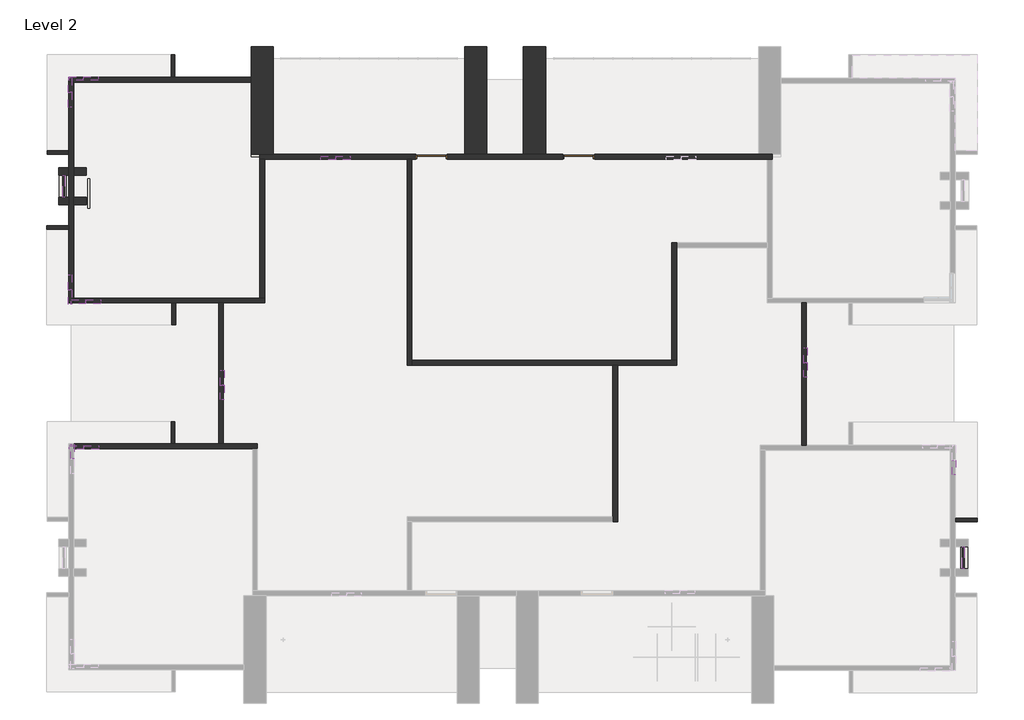
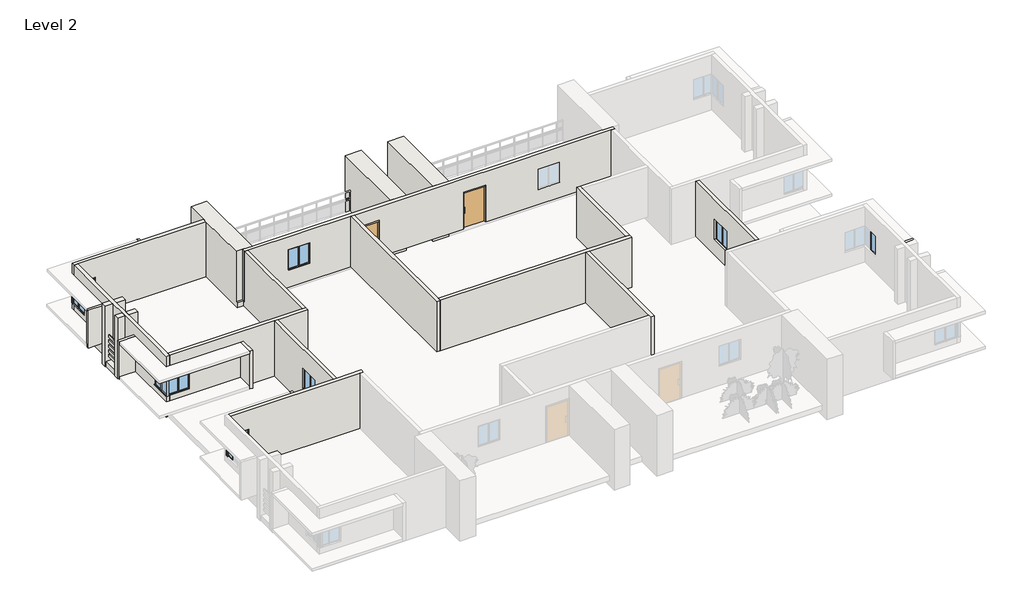
# One storey, part 2 of 4: 37 walls, 18 windows, 2 doors.
"""IFC4 building model written with IfcOpenShell, lengths in millimetres."""

from ifc_helpers import new_model, si_unit, frame, origin, place, context, project, spatial, polyline, outline, extrude, faceted_brep, transform, mapped, element, save
from components import door_15d3c954, window_20ff4747

model = new_model("IFC4")

# Units and contexts
model_context = context("Model", 3, world=origin())
ifc_project = project(units=[si_unit("LENGTHUNIT", "METRE", prefix="MILLI")], contexts=[model_context])

# Site, building, storey
site = spatial("IfcSite", under=ifc_project)
building = spatial("IfcBuilding", under=site)
storey = spatial("IfcBuildingStorey", under=building, Name="Level 2", Elevation=3048.0)

# Doors
placement = place(None, origin())
door_shape = door_15d3c954(model_context)
element("IfcDoor", 1, ObjectType="Door-Passage-Single-Flush-Dbl_Acting : 48\" x 96\"", at=placement, inside=storey, context=model_context, shape_type="MappedRepresentation", body=[
    mapped(door_shape, transform((6249.0520665, 12804.5205944, 3657.6), x_axis=(1.0, 0.0, 0.0), y_axis=(0.0, 1.0, 0.0), z_axis=(0.0, 0.0, 1.0))),
])
element("IfcDoor", 2, ObjectType="Door-Passage-Single-Flush-Dbl_Acting : 48\" x 96\"", at=placement, inside=storey, context=model_context, shape_type="MappedRepresentation", body=[
    mapped(door_shape, transform((153.0520665, 12804.5205944, 3657.6), x_axis=(1.0, 0.0, 0.0), y_axis=(0.0, 1.0, 0.0), z_axis=(0.0, 0.0, 1.0))),
])

# Walls
element("IfcWall", 3, ObjectType="Generic - 1'", at=placement, inside=storey, context=model_context, shape_type="SweptSolid", body=[
    extrude(outline(polyline([(-14151.7972154, 12048.8705944), (-14667.8479335, 12048.8705944), (-14667.8479335, 12353.6705944), (-14151.7972154, 12353.6705944), (-14151.7972154, 12048.8705944)])), frame((0.0, 0.0, 3048.0), z_axis=(0.0, 0.0, 1.0), x_axis=(1.0, 0.0, 0.0)), (0.0, 0.0, 1.0), 3657.6),
])
element("IfcWall", 4, ObjectType="Generic - 1'", at=placement, inside=storey, context=model_context, shape_type="Brep", body=[
    faceted_brep([(-14871.0479335, 12353.6705944, 3048.0), (-15302.1394029, 12353.6705944, 3048.0), (-15302.1394029, 12353.6705944, 6705.6), (-14871.0479335, 12353.6705944, 6705.6), (-14871.0479335, 12048.8705944, 3048.0), (-14871.0479335, 12048.8705944, 6705.6), (-15302.1394029, 12048.8705944, 6705.6), (-15302.1394029, 12048.8705944, 3048.0), (-15277.0936682, 12048.8705944, 3048.0), (-14972.2936682, 12048.8705944, 3048.0)], [[[0, 1, 2, 3]], [[4, 5, 6, 7, 8, 9]], [[1, 0, 4, 9, 8, 7]], [[2, 1, 7, 6]], [[3, 2, 6, 5]], [[0, 3, 5, 4]]]),
])
element("IfcWall", 5, ObjectType="Generic - 1'", at=placement, inside=storey, context=model_context, shape_type="SweptSolid", body=[
    extrude(outline(polyline([(-14151.7972154, 10829.6705944), (-14667.8479335, 10829.6705944), (-14667.8479335, 11134.4705944), (-14151.7972154, 11134.4705944), (-14151.7972154, 10829.6705944)])), frame((0.0, 0.0, 3048.0), z_axis=(0.0, 0.0, 1.0), x_axis=(1.0, 0.0, 0.0)), (0.0, 0.0, 1.0), 3657.6),
])
element("IfcWall", 6, ObjectType="Generic - 1'", at=placement, inside=storey, context=model_context, shape_type="Brep", body=[
    faceted_brep([(-14871.0479335, 11134.4705944, 3048.0), (-14972.2936682, 11134.4705944, 3048.0), (-15277.0936682, 11134.4705944, 3048.0), (-15302.1394029, 11134.4705944, 3048.0), (-15302.1394029, 11134.4705944, 6705.6), (-14871.0479335, 11134.4705944, 6705.6), (-14871.0479335, 10829.6705944, 3048.0), (-14871.0479335, 10829.6705944, 6705.6), (-15302.1394029, 10829.6705944, 6705.6), (-15302.1394029, 10829.6705944, 3048.0)], [[[0, 1, 2, 3, 4, 5]], [[6, 7, 8, 9]], [[3, 2, 1, 0, 6, 9]], [[4, 3, 9, 8]], [[5, 4, 8, 7]], [[0, 5, 7, 6]]]),
])
element("IfcWall", 7, ObjectType="Generic - 2'", at=placement, inside=storey, context=model_context, shape_type="SweptSolid", body=[
    extrude(outline(polyline([(22069.7857703, -4257.9294056), (22069.7857703, -3343.5294056), (22374.5857703, -3343.5294056), (22374.5857703, -4257.9294056), (22069.7857703, -4257.9294056)])), frame((0.0, 0.0, 3048.0), z_axis=(0.0, 0.0, 1.0), x_axis=(1.0, 0.0, 0.0)), (0.0, 0.0, 1.0), 304.8),
])
element("IfcWall", 8, ObjectType="Generic - 2'", at=placement, inside=storey, context=model_context, shape_type="SweptSolid", body=[
    extrude(outline(polyline([(-15277.0936682, 11134.4705944), (-15277.0936682, 12048.8705944), (-14972.2936682, 12048.8705944), (-14972.2936682, 11134.4705944), (-15277.0936682, 11134.4705944)])), frame((0.0, 0.0, 3048.0), z_axis=(0.0, 0.0, 1.0), x_axis=(1.0, 0.0, 0.0)), (0.0, 0.0, 1.0), 304.8),
])
element("IfcWall", 9, ObjectType="Generic - 3'", at=placement, inside=storey, context=model_context, shape_type="SweptSolid", body=[
    extrude(outline(polyline([(2439.0520665, 17382.8705944), (2439.0520665, 12912.4705944), (1524.6520665, 12912.4705944), (1524.6520665, 17382.8705944), (2439.0520665, 17382.8705944)])), frame((0.0, 0.0, 3048.0), z_axis=(0.0, 0.0, 1.0), x_axis=(1.0, 0.0, 0.0)), (0.0, 0.0, 1.0), 3657.6),
])
element("IfcWall", 10, ObjectType="Generic - 3'", at=placement, inside=storey, context=model_context, shape_type="SweptSolid", body=[
    extrude(outline(polyline([(4877.4520665, 17382.8705944), (4877.4520665, 12912.4705944), (3963.0520665, 12912.4705944), (3963.0520665, 17382.8705944), (4877.4520665, 17382.8705944)])), frame((0.0, 0.0, 3048.0), z_axis=(0.0, 0.0, 1.0), x_axis=(1.0, 0.0, 0.0)), (0.0, 0.0, 1.0), 3657.6),
])
element("IfcWall", 11, ObjectType="Generic - 3'", at=placement, inside=storey, context=model_context, shape_type="Brep", body=[
    faceted_brep([(-6400.1479335, 12810.8705944, 3048.0), (-6400.1479335, 17382.8705944, 3048.0), (-6400.1479335, 17382.8705944, 6705.6), (-6400.1479335, 12912.4705944, 6705.6), (-6400.1479335, 12912.4705944, 3657.6), (-6400.1479335, 12810.8705944, 3657.6), (-7314.5479335, 12810.8705944, 3048.0), (-7314.5479335, 12810.8705944, 3657.6), (-7314.5479335, 12912.4705944, 3657.6), (-7314.5479335, 12912.4705944, 6705.6), (-7314.5479335, 15904.9548886, 6705.6), (-7314.5479335, 16108.1548886, 6705.6), (-7314.5479335, 17382.8705944, 6705.6), (-7314.5479335, 17382.8705944, 3048.0), (-7314.5479335, 16108.1548886, 3048.0), (-7314.5479335, 15904.9548886, 3048.0), (-6755.7479335, 12810.8705944, 3048.0), (-6958.9479335, 12810.8705944, 3048.0), (-6958.9479335, 12912.4705944, 6705.6), (-6755.7479335, 12810.8705944, 3657.6), (-6958.9479335, 12810.8705944, 3657.6), (-6958.9479335, 12912.4705944, 3657.6)], [[[0, 1, 2, 3, 4, 5]], [[6, 7, 8, 9, 10, 11, 12, 13, 14, 15]], [[1, 0, 16, 17, 6, 15, 14, 13]], [[2, 1, 13, 12]], [[3, 2, 12, 11, 10, 9, 18]], [[0, 5, 19, 20, 7, 6, 17, 16]], [[4, 21, 8, 7, 20, 19, 5]], [[4, 3, 18, 9, 8, 21]]]),
])
element("IfcWall", 12, ObjectType="Generic - 5\"", at=placement, inside=storey, context=model_context, shape_type="SweptSolid", body=[
    extrude(outline(polyline([(-14084.4224108, 10677.2705944), (-14084.4224108, 11896.4705944), (-14008.2224108, 11896.4705944), (-14008.2224108, 10677.2705944), (-14084.4224108, 10677.2705944)])), frame((0.0, 0.0, 3302.0), z_axis=(0.0, 0.0, 1.0), x_axis=(1.0, 0.0, 0.0)), (0.0, 0.0, 1.0), 178.1810075),
])
element("IfcWall", 13, ObjectType="Generic - 5\"", at=placement, inside=storey, context=model_context, shape_type="SweptSolid", body=[
    extrude(outline(polyline([(-15124.6936682, 11134.4705944), (-15124.6936682, 12048.8705944), (-15048.4936682, 12048.8705944), (-15048.4936682, 11134.4705944), (-15124.6936682, 11134.4705944)])), frame((0.0, 0.0, 3581.4), z_axis=(0.0, 0.0, 1.0), x_axis=(1.0, 0.0, 0.0)), (0.0, 0.0, 1.0), 152.8735856),
])
element("IfcWall", 14, ObjectType="Generic - 5\"", at=placement, inside=storey, context=model_context, shape_type="SweptSolid", body=[
    extrude(outline(polyline([(-15124.6936682, 11134.4705944), (-15124.6936682, 12048.8705944), (-15048.4936682, 12048.8705944), (-15048.4936682, 11134.4705944), (-15124.6936682, 11134.4705944)])), frame((0.0, 0.0, 3860.8), z_axis=(0.0, 0.0, 1.0), x_axis=(1.0, 0.0, 0.0)), (0.0, 0.0, 1.0), 152.8735856),
])
element("IfcWall", 15, ObjectType="Generic - 5\"", at=placement, inside=storey, context=model_context, shape_type="SweptSolid", body=[
    extrude(outline(polyline([(-15124.6936682, 11134.4705944), (-15124.6936682, 12048.8705944), (-15048.4936682, 12048.8705944), (-15048.4936682, 11134.4705944), (-15124.6936682, 11134.4705944)])), frame((0.0, 0.0, 4165.6), z_axis=(0.0, 0.0, 1.0), x_axis=(1.0, 0.0, 0.0)), (0.0, 0.0, 1.0), 152.8735856),
])
element("IfcWall", 16, ObjectType="Generic - 5\"", at=placement, inside=storey, context=model_context, shape_type="SweptSolid", body=[
    extrude(outline(polyline([(-15124.6936682, 11134.4705944), (-15124.6936682, 12048.8705944), (-15048.4936682, 12048.8705944), (-15048.4936682, 11134.4705944), (-15124.6936682, 11134.4705944)])), frame((0.0, 0.0, 4470.4), z_axis=(0.0, 0.0, 1.0), x_axis=(1.0, 0.0, 0.0)), (0.0, 0.0, 1.0), 152.8735856),
])
element("IfcWall", 17, ObjectType="Generic - 5\"", at=placement, inside=storey, context=model_context, shape_type="SweptSolid", body=[
    extrude(outline(polyline([(-15124.6936682, 11134.4705944), (-15124.6936682, 12048.8705944), (-15048.4936682, 12048.8705944), (-15048.4936682, 11134.4705944), (-15124.6936682, 11134.4705944)])), frame((0.0, 0.0, 4749.8), z_axis=(0.0, 0.0, 1.0), x_axis=(1.0, 0.0, 0.0)), (0.0, 0.0, 1.0), 152.8735856),
])
element("IfcWall", 18, ObjectType="Generic - 5\"", at=placement, inside=storey, context=model_context, shape_type="SweptSolid", body=[
    extrude(outline(polyline([(22145.9857703, -4257.9294056), (22145.9857703, -3343.5294056), (22222.1857703, -3343.5294056), (22222.1857703, -4257.9294056), (22145.9857703, -4257.9294056)])), frame((0.0, 0.0, 3860.8), z_axis=(0.0, 0.0, 1.0), x_axis=(1.0, 0.0, 0.0)), (0.0, 0.0, 1.0), 152.8735856),
])
element("IfcWall", 19, ObjectType="Generic - 5\"", at=placement, inside=storey, context=model_context, shape_type="SweptSolid", body=[
    extrude(outline(polyline([(22145.9857703, -4257.9294056), (22145.9857703, -3343.5294056), (22222.1857703, -3343.5294056), (22222.1857703, -4257.9294056), (22145.9857703, -4257.9294056)])), frame((0.0, 0.0, 4165.6), z_axis=(0.0, 0.0, 1.0), x_axis=(1.0, 0.0, 0.0)), (0.0, 0.0, 1.0), 152.8735856),
])
element("IfcWall", 20, ObjectType="Generic - 5\"", at=placement, inside=storey, context=model_context, shape_type="SweptSolid", body=[
    extrude(outline(polyline([(22145.9857703, -4257.9294056), (22145.9857703, -3343.5294056), (22222.1857703, -3343.5294056), (22222.1857703, -4257.9294056), (22145.9857703, -4257.9294056)])), frame((0.0, 0.0, 4470.4), z_axis=(0.0, 0.0, 1.0), x_axis=(1.0, 0.0, 0.0)), (0.0, 0.0, 1.0), 152.8735856),
])
element("IfcWall", 21, ObjectType="Generic - 5\"", at=placement, inside=storey, context=model_context, shape_type="SweptSolid", body=[
    extrude(outline(polyline([(22145.9857703, -4257.9294056), (22145.9857703, -3343.5294056), (22222.1857703, -3343.5294056), (22222.1857703, -4257.9294056), (22145.9857703, -4257.9294056)])), frame((0.0, 0.0, 4749.8), z_axis=(0.0, 0.0, 1.0), x_axis=(1.0, 0.0, 0.0)), (0.0, 0.0, 1.0), 152.8735856),
])
element("IfcWall", 22, ObjectType="Generic - 6\"", at=placement, inside=storey, context=model_context, shape_type="SweptSolid", body=[
    extrude(outline(polyline([(-10480.7034654, 17035.2548886), (-10480.7034654, 16120.8548886), (-10633.1034654, 16120.8548886), (-10633.1034654, 17035.2548886), (-10480.7034654, 17035.2548886)])), frame((0.0, 0.0, 3810.0), z_axis=(0.0, 0.0, 1.0), x_axis=(1.0, 0.0, 0.0)), (0.0, 0.0, 1.0), 2286.0),
])
element("IfcWall", 23, ObjectType="Generic - 6\"", at=placement, inside=storey, context=model_context, shape_type="SweptSolid", body=[
    extrude(outline(polyline([(-15775.8097154, 13072.8548886), (-14883.7479335, 13072.8548886), (-14883.7479335, 12920.4548886), (-15775.8097154, 12920.4548886), (-15775.8097154, 13072.8548886)])), frame((0.0, 0.0, 3810.0), z_axis=(0.0, 0.0, 1.0), x_axis=(1.0, 0.0, 0.0)), (0.0, 0.0, 1.0), 2286.0),
])
element("IfcWall", 24, ObjectType="Generic - 6\"", at=placement, inside=storey, context=model_context, shape_type="SweptSolid", body=[
    extrude(outline(polyline([(-10603.8479335, 5846.5548886), (-10603.8479335, 6760.9548886), (-10451.4479335, 6760.9548886), (-10451.4479335, 5846.5548886), (-10603.8479335, 5846.5548886)])), frame((0.0, 0.0, 3810.0), z_axis=(0.0, 0.0, 1.0), x_axis=(1.0, 0.0, 0.0)), (0.0, 0.0, 1.0), 2286.0),
])
element("IfcWall", 25, ObjectType="Generic - 6\"", at=placement, inside=storey, context=model_context, shape_type="SweptSolid", body=[
    extrude(outline(polyline([(-15798.1479335, 9961.3548886), (-14883.7479335, 9961.3548886), (-14883.7479335, 9808.9548886), (-15798.1479335, 9808.9548886), (-15798.1479335, 9961.3548886)])), frame((0.0, 0.0, 3810.0), z_axis=(0.0, 0.0, 1.0), x_axis=(1.0, 0.0, 0.0)), (0.0, 0.0, 1.0), 2286.0),
])
element("IfcWall", 26, ObjectType="Generic - 6\"", at=placement, inside=storey, context=model_context, shape_type="SweptSolid", body=[
    extrude(outline(polyline([(-10480.7034654, 1834.0395301), (-10480.7034654, 919.6395301), (-10633.1034654, 919.6395301), (-10633.1034654, 1834.0395301), (-10480.7034654, 1834.0395301)])), frame((0.0, 0.0, 3810.0), z_axis=(0.0, 0.0, 1.0), x_axis=(1.0, 0.0, 0.0)), (0.0, 0.0, 1.0), 2286.0),
])
element("IfcWall", 27, ObjectType="Generic - 6\"", at=placement, inside=storey, context=model_context, shape_type="SweptSolid", body=[
    extrude(outline(polyline([(22771.7520665, -2309.5899195), (21857.3520665, -2309.5899195), (21857.3520665, -2157.1899195), (22771.7520665, -2157.1899195), (22771.7520665, -2309.5899195)])), frame((0.0, 0.0, 3810.0), z_axis=(0.0, 0.0, 1.0), x_axis=(1.0, 0.0, 0.0)), (0.0, 0.0, 1.0), 2286.0),
])
element("IfcWall", 28, ObjectType="Generic - 8\"", at=placement, inside=storey, context=model_context, shape_type="Brep", body=[
    faceted_brep([(-862.9479335, 12709.2705944, 3657.6), (-862.9479335, 4174.8705944, 3657.6), (-862.9479335, 4174.8705944, 6705.6), (-862.9479335, 12709.2705944, 6705.6), (-659.7479335, 12709.2705944, 3657.6), (-659.7479335, 12709.2705944, 6705.6), (-659.7479335, 4378.0705944, 6705.6), (-659.7479335, 4174.8705944, 6705.6), (-659.7479335, 4174.8705944, 3657.6), (-659.7479335, 4378.0705944, 3657.6)], [[[0, 1, 2, 3]], [[4, 5, 6, 7, 8, 9]], [[1, 0, 4, 9, 8]], [[3, 2, 7, 6, 5]], [[0, 3, 5, 4]], [[2, 1, 8, 7]]]),
])
element("IfcWall", 29, ObjectType="Generic - 8\"", at=placement, inside=storey, context=model_context, shape_type="Brep", body=[
    faceted_brep([(-659.7479335, 4174.8705944, 3657.6), (7671.4520665, 4174.8705944, 3657.6), (7874.6520665, 4174.8705944, 3657.6), (10313.0520665, 4174.8705944, 3657.6), (10313.0520665, 4174.8705944, 6705.6), (7874.6520665, 4174.8705944, 6705.6), (7671.4520665, 4174.8705944, 6705.6), (-659.7479335, 4174.8705944, 6705.6), (-659.7479335, 4378.0705944, 3657.6), (-659.7479335, 4378.0705944, 6705.6), (10109.8520665, 4378.0705944, 6705.6), (10313.0520665, 4378.0705944, 6705.6), (10313.0520665, 4378.0705944, 3657.6), (10109.8520665, 4378.0705944, 3657.6)], [[[0, 1, 2, 3, 4, 5, 6, 7]], [[8, 9, 10, 11, 12, 13]], [[3, 2, 1, 0, 8, 13, 12]], [[7, 6, 5, 4, 11, 10, 9]], [[0, 7, 9, 8]], [[4, 3, 12, 11]]]),
])
element("IfcWall", 30, ObjectType="Generic - 8\"", at=placement, inside=storey, context=model_context, shape_type="Brep", body=[
    faceted_brep([(10313.0520665, 4378.0705944, 3657.6), (10313.0520665, 9051.6705944, 3657.6), (10313.0520665, 9254.8705944, 3657.6), (10313.0520665, 9254.8705944, 6705.6), (10313.0520665, 9051.6705944, 6705.6), (10313.0520665, 4378.0705944, 6705.6), (10109.8520665, 4378.0705944, 3657.6), (10109.8520665, 4378.0705944, 6705.6), (10109.8520665, 9254.8705944, 6705.6), (10109.8520665, 9254.8705944, 3657.6)], [[[0, 1, 2, 3, 4, 5]], [[6, 7, 8, 9]], [[2, 1, 0, 6, 9]], [[5, 4, 3, 8, 7]], [[0, 5, 7, 6]], [[3, 2, 9, 8]]]),
])
element("IfcWall", 31, ObjectType="Generic - 8\"", at=placement, inside=storey, context=model_context, shape_type="Brep", body=[
    faceted_brep([(7671.4520665, 4174.8705944, 3657.6), (7671.4520665, -2102.9604699, 3657.6), (7671.4520665, -2306.1604699, 3657.6), (7671.4520665, -2306.1604699, 6705.6), (7671.4520665, -2102.9604699, 6705.6), (7671.4520665, 4174.8705944, 6705.6), (7874.6520665, 4174.8705944, 3657.6), (7874.6520665, 4174.8705944, 6705.6), (7874.6520665, -2306.1604699, 6705.6), (7874.6520665, -2306.1604699, 3657.6)], [[[0, 1, 2, 3, 4, 5]], [[6, 7, 8, 9]], [[2, 1, 0, 6, 9]], [[5, 4, 3, 8, 7]], [[0, 5, 7, 6]], [[3, 2, 9, 8]]]),
])
element("IfcWall", 32, ObjectType="Generic - 8\" gray", at=placement, inside=storey, context=model_context, shape_type="Brep", body=[
    faceted_brep([(-14871.0479335, 15904.9548886, 3048.0), (-14667.8479335, 15904.9548886, 3048.0), (-7314.5479335, 15904.9548886, 3048.0), (-7314.5479335, 15904.9548886, 6705.6), (-14667.8479335, 15904.9548886, 6705.6), (-14871.0479335, 15904.9548886, 6705.6), (-14871.0479335, 15904.9548886, 5539.4804451), (-14667.8479335, 15904.9548886, 5539.4804451), (-13661.292575, 15904.9548886, 5539.4804451), (-13661.292575, 15904.9548886, 4320.2804451), (-14667.8479335, 15904.9548886, 4320.2804451), (-14871.0479335, 15904.9548886, 4320.2804451), (-7314.5479335, 16108.1548886, 3048.0), (-14871.0479335, 16108.1548886, 3048.0), (-14871.0479335, 16108.1548886, 4320.2804451), (-13661.292575, 16108.1548886, 4320.2804451), (-13661.292575, 16108.1548886, 5539.4804451), (-14871.0479335, 16108.1548886, 5539.4804451), (-14871.0479335, 16108.1548886, 6705.6), (-7314.5479335, 16108.1548886, 6705.6)], [[[0, 1, 2, 3, 4, 5, 6, 7, 8, 9, 10, 11]], [[12, 13, 14, 15, 16, 17, 18, 19]], [[2, 1, 0, 13, 12]], [[5, 4, 3, 19, 18]], [[5, 18, 17, 6]], [[13, 0, 11, 14]], [[3, 2, 12, 19]], [[9, 15, 14, 11, 10]], [[6, 17, 16, 8, 7]], [[8, 16, 15, 9]]]),
])
element("IfcWall", 33, ObjectType="Generic - 8\" gray", at=placement, inside=storey, context=model_context, shape_type="Brep", body=[
    faceted_brep([(-14667.8479335, 6760.9548886, 3048.0), (-14667.8479335, 6964.1548886, 3048.0), (-14667.8479335, 10829.6705944, 3048.0), (-14667.8479335, 11134.4705944, 3048.0), (-14667.8479335, 12048.8705944, 3048.0), (-14667.8479335, 12353.6705944, 3048.0), (-14667.8479335, 15904.9548886, 3048.0), (-14667.8479335, 15904.9548886, 4320.2804451), (-14667.8479335, 14871.0236266, 4320.2804451), (-14667.8479335, 14871.0236266, 5539.4804451), (-14667.8479335, 15904.9548886, 5539.4804451), (-14667.8479335, 15904.9548886, 6705.6), (-14667.8479335, 12353.6705944, 6705.6), (-14667.8479335, 12048.8705944, 6705.6), (-14667.8479335, 11134.4705944, 6705.6), (-14667.8479335, 10829.6705944, 6705.6), (-14667.8479335, 6964.1548886, 6705.6), (-14667.8479335, 6760.9548886, 6705.6), (-14667.8479335, 6760.9548886, 5539.4804451), (-14667.8479335, 6964.1548886, 5539.4804451), (-14667.8479335, 7918.4820466, 5539.4804451), (-14667.8479335, 7918.4820466, 4320.2804451), (-14667.8479335, 6964.1548886, 4320.2804451), (-14667.8479335, 6760.9548886, 4320.2804451), (-14871.0479335, 15904.9548886, 3048.0), (-14871.0479335, 12353.6705944, 3048.0), (-14871.0479335, 12048.8705944, 3048.0), (-14871.0479335, 11134.4705944, 3048.0), (-14871.0479335, 10829.6705944, 3048.0), (-14871.0479335, 6760.9548886, 3048.0), (-14871.0479335, 6760.9548886, 4320.2804451), (-14871.0479335, 7918.4820466, 4320.2804451), (-14871.0479335, 7918.4820466, 5539.4804451), (-14871.0479335, 6760.9548886, 5539.4804451), (-14871.0479335, 6760.9548886, 6705.6), (-14871.0479335, 10829.6705944, 6705.6), (-14871.0479335, 11134.4705944, 6705.6), (-14871.0479335, 12048.8705944, 6705.6), (-14871.0479335, 12353.6705944, 6705.6), (-14871.0479335, 15904.9548886, 6705.6), (-14871.0479335, 15904.9548886, 5539.4804451), (-14871.0479335, 14871.0236266, 5539.4804451), (-14871.0479335, 14871.0236266, 4320.2804451), (-14871.0479335, 15904.9548886, 4320.2804451)], [[[0, 1, 2, 3, 4, 5, 6, 7, 8, 9, 10, 11, 12, 13, 14, 15, 16, 17, 18, 19, 20, 21, 22, 23]], [[24, 25, 26, 27, 28, 29, 30, 31, 32, 33, 34, 35, 36, 37, 38, 39, 40, 41, 42, 43]], [[6, 5, 4, 3, 2, 1, 0, 29, 28, 27, 26, 25, 24]], [[17, 16, 15, 14, 13, 12, 11, 39, 38, 37, 36, 35, 34]], [[17, 34, 33, 18]], [[29, 0, 23, 30]], [[6, 24, 43, 7]], [[39, 11, 10, 40]], [[30, 23, 22, 21, 31]], [[18, 33, 32, 20, 19]], [[20, 32, 31, 21]], [[7, 43, 42, 8]], [[9, 8, 42, 41]], [[9, 41, 40, 10]]]),
])
element("IfcWall", 34, ObjectType="Generic - 8\" gray", at=placement, inside=storey, context=model_context, shape_type="Brep", body=[
    faceted_brep([(-6755.7479335, 6964.1548886, 3048.0), (-6958.9479335, 6964.1548886, 3048.0), (-14667.8479335, 6964.1548886, 3048.0), (-14667.8479335, 6964.1548886, 4320.2804451), (-13556.3228261, 6964.1548886, 4320.2804451), (-13556.3228261, 6964.1548886, 5539.4804451), (-14667.8479335, 6964.1548886, 5539.4804451), (-14667.8479335, 6964.1548886, 6705.6), (-6958.9479335, 6964.1548886, 6705.6), (-6755.7479335, 6964.1548886, 6705.6), (-14667.8479335, 6760.9548886, 3048.0), (-8673.4479335, 6760.9548886, 3048.0), (-8470.2479335, 6760.9548886, 3048.0), (-6755.7479335, 6760.9548886, 3048.0), (-6755.7479335, 6760.9548886, 6705.6), (-8470.2479335, 6760.9548886, 6705.6), (-8673.4479335, 6760.9548886, 6705.6), (-14667.8479335, 6760.9548886, 6705.6), (-14667.8479335, 6760.9548886, 5539.4804451), (-13556.3228261, 6760.9548886, 5539.4804451), (-13556.3228261, 6760.9548886, 4320.2804451), (-14667.8479335, 6760.9548886, 4320.2804451)], [[[0, 1, 2, 3, 4, 5, 6, 7, 8, 9]], [[10, 11, 12, 13, 14, 15, 16, 17, 18, 19, 20, 21]], [[2, 1, 0, 13, 12, 11, 10]], [[9, 8, 7, 17, 16, 15, 14]], [[2, 10, 21, 3]], [[17, 7, 6, 18]], [[0, 9, 14, 13]], [[3, 21, 20, 4]], [[5, 4, 20, 19]], [[5, 19, 18, 6]]]),
])
element("IfcWall", 35, ObjectType="Generic - 8\" gray", at=placement, inside=storey, context=model_context, shape_type="Brep", body=[
    faceted_brep([(-7060.5479335, 919.6395301, 3048.0), (-8470.2479335, 919.6395301, 3048.0), (-8673.4479335, 919.6395301, 3048.0), (-14680.5479335, 919.6395301, 3048.0), (-14680.5479335, 919.6395301, 4320.2804451), (-13641.9760869, 919.6395301, 4320.2804451), (-13641.9760869, 919.6395301, 5539.4804451), (-14680.5479335, 919.6395301, 5539.4804451), (-14680.5479335, 919.6395301, 6705.6), (-8673.4479335, 919.6395301, 6705.6), (-8470.2479335, 919.6395301, 6705.6), (-7060.5479335, 919.6395301, 6705.6), (-14680.5479335, 716.4395301, 3048.0), (-7263.7479335, 716.4395301, 3048.0), (-7060.5479335, 716.4395301, 3048.0), (-7060.5479335, 716.4395301, 6705.6), (-7263.7479335, 716.4395301, 6705.6), (-14680.5479335, 716.4395301, 6705.6), (-14680.5479335, 716.4395301, 5539.4804451), (-13641.9760869, 716.4395301, 5539.4804451), (-13641.9760869, 716.4395301, 4320.2804451), (-14680.5479335, 716.4395301, 4320.2804451), (-14680.5479335, 908.9135189, 4320.2804451), (-14680.5479335, 908.9135189, 5539.4804451)], [[[0, 1, 2, 3, 4, 5, 6, 7, 8, 9, 10, 11]], [[12, 13, 14, 15, 16, 17, 18, 19, 20, 21]], [[3, 2, 1, 0, 14, 13, 12]], [[11, 10, 9, 8, 17, 16, 15]], [[3, 12, 21, 22, 4]], [[17, 8, 7, 23, 18]], [[0, 11, 15, 14]], [[4, 22, 21, 20, 5]], [[6, 5, 20, 19]], [[6, 19, 18, 23, 7]]]),
])
element("IfcWall", 36, ObjectType="Generic - 8\" gray", at=placement, inside=storey, context=model_context, shape_type="SweptSolid", body=[
    extrude(outline(polyline([(6760.9548886, 3048.0), (919.6395301, 3048.0), (919.6395301, 6705.6), (6760.9548886, 6705.6), (6760.9548886, 3048.0)]), holes=[polyline([(2742.9076732, 4320.2804451), (3962.1076732, 4320.2804451), (3962.1076732, 5539.4804451), (2742.9076732, 5539.4804451), (2742.9076732, 4320.2804451)])]), frame((-8673.4479335, 0.0, 0.0), z_axis=(1.0, 0.0, 0.0), x_axis=(0.0, 1.0, 0.0)), (0.0, 0.0, 1.0), 203.2),
])
element("IfcWall", 37, ObjectType="Generic - 8\" gray", at=placement, inside=storey, context=model_context, shape_type="SweptSolid", body=[
    extrude(outline(polyline([(6760.9548886, 3048.0), (868.1548886, 3048.0), (868.1548886, 6705.6), (6760.9548886, 6705.6), (6760.9548886, 3048.0)]), holes=[polyline([(3676.3636585, 4320.2804451), (4895.5636585, 4320.2804451), (4895.5636585, 5539.4804451), (3676.3636585, 5539.4804451), (3676.3636585, 4320.2804451)])]), frame((15481.9520665, 0.0, 0.0), z_axis=(1.0, 0.0, 0.0), x_axis=(0.0, 1.0, 0.0)), (0.0, 0.0, 1.0), 203.2),
])
element("IfcWall", 38, ObjectType="Generic - 8\" gray", at=placement, inside=storey, context=model_context, shape_type="Brep", body=[
    faceted_brep([(-6958.9479335, 12912.4705944, 6705.6), (-6400.1479335, 12912.4705944, 6705.6), (1524.6520665, 12912.4705944, 6705.6), (2439.0520665, 12912.4705944, 6705.6), (3963.0520665, 12912.4705944, 6705.6), (4877.4520665, 12912.4705944, 6705.6), (13716.6520665, 12912.4705944, 6705.6), (14275.4520665, 12912.4705944, 6705.6), (14275.4520665, 12912.4705944, 3657.6), (13716.6520665, 12912.4705944, 3657.6), (6909.4520665, 12912.4705944, 3657.6), (6909.4520665, 12912.4705944, 5892.8), (5588.6520665, 12912.4705944, 5892.8), (5588.6520665, 12912.4705944, 3657.6), (813.4520665, 12912.4705944, 3657.6), (813.4520665, 12912.4705944, 5892.8), (-507.3479335, 12912.4705944, 5892.8), (-507.3479335, 12912.4705944, 3657.6), (-6400.1479335, 12912.4705944, 3657.6), (-6958.9479335, 12912.4705944, 3657.6), (11102.1500799, 12912.4705944, 4576.8873953), (11102.1500799, 12912.4705944, 5796.0873953), (9882.9500799, 12912.4705944, 5796.0873953), (9882.9500799, 12912.4705944, 4576.8873953), (-3213.321881, 12912.4705944, 4703.0298362), (-3213.321881, 12912.4705944, 5922.2298362), (-4432.521881, 12912.4705944, 5922.2298362), (-4432.521881, 12912.4705944, 4703.0298362), (14275.4520665, 12709.2705944, 6705.6), (14072.2520665, 12709.2705944, 6705.6), (-659.7479335, 12709.2705944, 6705.6), (-862.9479335, 12709.2705944, 6705.6), (-6755.7479335, 12709.2705944, 6705.6), (-6958.9479335, 12709.2705944, 6705.6), (-6958.9479335, 12709.2705944, 3657.6), (-6755.7479335, 12709.2705944, 3657.6), (-862.9479335, 12709.2705944, 3657.6), (-659.7479335, 12709.2705944, 3657.6), (-507.3479335, 12709.2705944, 3657.6), (-507.3479335, 12709.2705944, 5892.8), (813.4520665, 12709.2705944, 5892.8), (813.4520665, 12709.2705944, 3657.6), (5588.6520665, 12709.2705944, 3657.6), (5588.6520665, 12709.2705944, 5892.8), (6909.4520665, 12709.2705944, 5892.8), (6909.4520665, 12709.2705944, 3657.6), (14072.2520665, 12709.2705944, 3657.6), (14275.4520665, 12709.2705944, 3657.6), (11102.1500799, 12709.2705944, 5796.0873953), (11102.1500799, 12709.2705944, 4576.8873953), (9882.9500799, 12709.2705944, 4576.8873953), (9882.9500799, 12709.2705944, 5796.0873953), (-3213.321881, 12709.2705944, 5922.2298362), (-3213.321881, 12709.2705944, 4703.0298362), (-4432.521881, 12709.2705944, 4703.0298362), (-4432.521881, 12709.2705944, 5922.2298362), (14275.4520665, 12810.8705944, 3657.6), (-6958.9479335, 12810.8705944, 3657.6)], [[[0, 1, 2, 3, 4, 5, 6, 7, 8, 9, 10, 11, 12, 13, 14, 15, 16, 17, 18, 19], [20, 21, 22, 23], [24, 25, 26, 27]], [[28, 29, 30, 31, 32, 33, 34, 35, 36, 37, 38, 39, 40, 41, 42, 43, 44, 45, 46, 47], [48, 49, 50, 51], [52, 53, 54, 55]], [[8, 56, 47, 46, 45, 10, 9]], [[34, 57, 19, 18, 17, 38, 37, 36, 35]], [[13, 42, 41, 14]], [[7, 6, 5, 4, 3, 2, 1, 0, 33, 32, 31, 30, 29, 28]], [[8, 7, 28, 47, 56]], [[0, 19, 57, 34, 33]], [[49, 20, 23, 50]], [[21, 20, 49, 48]], [[21, 48, 51, 22]], [[22, 51, 50, 23]], [[53, 24, 27, 54]], [[25, 24, 53, 52]], [[25, 52, 55, 26]], [[26, 55, 54, 27]], [[44, 11, 10, 45]], [[11, 44, 43, 12]], [[12, 43, 42, 13]], [[40, 15, 14, 41]], [[15, 40, 39, 16]], [[16, 39, 38, 17]]]),
])
element("IfcWall", 39, ObjectType="Generic - 8\" gray", at=placement, inside=storey, context=model_context, shape_type="SweptSolid", body=[
    extrude(outline(polyline([(6964.1548886, 3048.0), (6964.1548886, 6705.6), (12709.2705944, 6705.6), (12709.2705944, 3657.6), (12810.8705944, 3657.6), (12810.8705944, 3048.0), (6964.1548886, 3048.0)])), frame((-6958.9479335, 0.0, 0.0), z_axis=(1.0, 0.0, 0.0), x_axis=(0.0, 1.0, 0.0)), (0.0, 0.0, 1.0), 203.2),
])

# Windows
window_shape = window_20ff4747(model_context)
element("IfcWindow", 40, ObjectType="Instance - Fixed : 24\" x 48\"", at=placement, inside=storey, context=model_context, shape_type="MappedRepresentation", body=[
    mapped(window_shape, transform((21755.7520665, -93.135515, 3405.8804451), x_axis=(0.0, -1.0, 0.0), y_axis=(1.0, 0.0, 0.0), z_axis=(0.0, 0.0, 1.0))),
])
element("IfcWindow", 41, ObjectType="Instance - Fixed : 24\" x 48\"", at=placement, inside=storey, context=model_context, shape_type="MappedRepresentation", body=[
    mapped(window_shape, transform((-14782.1479335, 566.0135189, 3405.8804451), x_axis=(0.0, -1.0, 0.0), y_axis=(1.0, 0.0, 0.0), z_axis=(0.0, 0.0, 1.0))),
])
element("IfcWindow", 42, ObjectType="Instance - Fixed : 24\" x 48\"", at=placement, inside=storey, context=model_context, shape_type="MappedRepresentation", body=[
    mapped(window_shape, transform((-14594.4760869, 818.0395301, 3405.8804451), x_axis=(-1.0, 0.0, 0.0), y_axis=(0.0, -1.0, 0.0), z_axis=(0.0, 0.0, 1.0))),
])
element("IfcWindow", 43, ObjectType="Instance - Fixed : 24\" x 48\"", at=placement, inside=storey, context=model_context, shape_type="MappedRepresentation", body=[
    mapped(window_shape, transform((-13984.8760869, 818.0395301, 3405.8804451), x_axis=(-1.0, 0.0, 0.0), y_axis=(0.0, -1.0, 0.0), z_axis=(0.0, 0.0, 1.0))),
])
element("IfcWindow", 44, ObjectType="Instance - Fixed : 24\" x 48\"", at=placement, inside=storey, context=model_context, shape_type="MappedRepresentation", body=[
    mapped(window_shape, transform((-14508.8228261, 6862.5548886, 3405.8804451), x_axis=(-1.0, 0.0, 0.0), y_axis=(0.0, -1.0, 0.0), z_axis=(0.0, 0.0, 1.0))),
])
element("IfcWindow", 45, ObjectType="Instance - Fixed : 24\" x 48\"", at=placement, inside=storey, context=model_context, shape_type="MappedRepresentation", body=[
    mapped(window_shape, transform((-13899.2228261, 6862.5548886, 3405.8804451), x_axis=(-1.0, 0.0, 0.0), y_axis=(0.0, -1.0, 0.0), z_axis=(0.0, 0.0, 1.0))),
])
element("IfcWindow", 46, ObjectType="Instance - Fixed : 24\" x 48\"", at=placement, inside=storey, context=model_context, shape_type="MappedRepresentation", body=[
    mapped(window_shape, transform((-14769.4479335, 7651.7820466, 3405.8804451), x_axis=(0.0, 1.0, 0.0), y_axis=(-1.0, 0.0, 0.0), z_axis=(0.0, 0.0, 1.0))),
])
element("IfcWindow", 47, ObjectType="Instance - Fixed : 24\" x 48\"", at=placement, inside=storey, context=model_context, shape_type="MappedRepresentation", body=[
    mapped(window_shape, transform((-14769.4479335, 7042.1820466, 3405.8804451), x_axis=(0.0, 1.0, 0.0), y_axis=(-1.0, 0.0, 0.0), z_axis=(0.0, 0.0, 1.0))),
])
element("IfcWindow", 48, ObjectType="Instance - Fixed : 24\" x 48\"", at=placement, inside=storey, context=model_context, shape_type="MappedRepresentation", body=[
    mapped(window_shape, transform((-14769.4479335, 15823.5236266, 3405.8804451), x_axis=(0.0, 1.0, 0.0), y_axis=(-1.0, 0.0, 0.0), z_axis=(0.0, 0.0, 1.0))),
])
element("IfcWindow", 49, ObjectType="Instance - Fixed : 24\" x 48\"", at=placement, inside=storey, context=model_context, shape_type="MappedRepresentation", body=[
    mapped(window_shape, transform((-14769.4479335, 15213.9236266, 3405.8804451), x_axis=(0.0, 1.0, 0.0), y_axis=(-1.0, 0.0, 0.0), z_axis=(0.0, 0.0, 1.0))),
])
element("IfcWindow", 50, ObjectType="Instance - Fixed : 24\" x 48\"", at=placement, inside=storey, context=model_context, shape_type="MappedRepresentation", body=[
    mapped(window_shape, transform((-13927.992575, 16006.5548886, 3405.8804451), x_axis=(1.0, 0.0, 0.0), y_axis=(0.0, 1.0, 0.0), z_axis=(0.0, 0.0, 1.0))),
])
element("IfcWindow", 51, ObjectType="Instance - Fixed : 24\" x 48\"", at=placement, inside=storey, context=model_context, shape_type="MappedRepresentation", body=[
    mapped(window_shape, transform((-14537.592575, 16006.5548886, 3405.8804451), x_axis=(1.0, 0.0, 0.0), y_axis=(0.0, 1.0, 0.0), z_axis=(0.0, 0.0, 1.0))),
])
element("IfcWindow", 52, ObjectType="Instance - Fixed : 24\" x 48\"", at=placement, inside=storey, context=model_context, shape_type="MappedRepresentation", body=[
    mapped(window_shape, transform((-4165.821881, 12810.8705944, 3788.6298362), x_axis=(-1.0, 0.0, 0.0), y_axis=(0.0, -1.0, 0.0), z_axis=(0.0, 0.0, 1.0))),
])
element("IfcWindow", 53, ObjectType="Instance - Fixed : 24\" x 48\"", at=placement, inside=storey, context=model_context, shape_type="MappedRepresentation", body=[
    mapped(window_shape, transform((-3556.221881, 12810.8705944, 3788.6298362), x_axis=(-1.0, 0.0, 0.0), y_axis=(0.0, -1.0, 0.0), z_axis=(0.0, 0.0, 1.0))),
])
element("IfcWindow", 54, ObjectType="Instance - Fixed : 24\" x 48\"", at=placement, inside=storey, context=model_context, shape_type="MappedRepresentation", body=[
    mapped(window_shape, transform((-8571.8479335, 3009.6076732, 3405.8804451), x_axis=(0.0, -1.0, 0.0), y_axis=(1.0, 0.0, 0.0), z_axis=(0.0, 0.0, 1.0))),
])
element("IfcWindow", 55, ObjectType="Instance - Fixed : 24\" x 48\"", at=placement, inside=storey, context=model_context, shape_type="MappedRepresentation", body=[
    mapped(window_shape, transform((-8571.8479335, 3619.2076732, 3405.8804451), x_axis=(0.0, -1.0, 0.0), y_axis=(1.0, 0.0, 0.0), z_axis=(0.0, 0.0, 1.0))),
])
element("IfcWindow", 56, ObjectType="Instance - Fixed : 24\" x 48\"", at=placement, inside=storey, context=model_context, shape_type="MappedRepresentation", body=[
    mapped(window_shape, transform((15583.5520665, 3943.0636585, 3405.8804451), x_axis=(0.0, -1.0, 0.0), y_axis=(1.0, 0.0, 0.0), z_axis=(0.0, 0.0, 1.0))),
])
element("IfcWindow", 57, ObjectType="Instance - Fixed : 24\" x 48\"", at=placement, inside=storey, context=model_context, shape_type="MappedRepresentation", body=[
    mapped(window_shape, transform((15583.5520665, 4552.6636585, 3405.8804451), x_axis=(0.0, -1.0, 0.0), y_axis=(1.0, 0.0, 0.0), z_axis=(0.0, 0.0, 1.0))),
])

save(model, "model.ifc")

# Revit data of these elements
# Type "Door-Passage-Single-Flush-Dbl_Acting : 48\" x 96\""
#   Type Mark = "12"
#   Assembly Code = "B2030200"
#   Analytic Construction = "Wooden"
#   Thickness = 0' - 1 3/4"
#   Thermal Resistance (R) = 2.5876 (h·ft²·°F)/BTU
#   Swing Angle [instance default] = 45.00°
#   Strike Height = 3' - 4"
#   Rough Width [instance default] = 4' - 4"
#   Rough Height [instance default] = 7' - 4"
#   MF Opening Height [instance default] = 0' - 4"
#   MF Opening Width [instance default] = 0' - 4"
#   Inset Calculate [instance default] = 0' - 4"
#   Masonry Inset [instance default] = 0' - 1"
#   Height = 7' - 0"
#   Width = 4' - 0"
#   Heat Transfer Coefficient (U) = 0.3865 BTU/(h·ft²·°F)
#   Masonry Frame Depth = 0' - 5 3/4"
#   Masonry Frame [instance default] = yes
#   Function = 1
#   Dry Wall Frame [instance default] = no
#   Panel Material = Wood - Birch
#   Frame Material = Metal - Paint Finish - Grey
#   Door Handle Material = Aluminum
#   Visual Light Transmittance = 0
#   Solar Heat Gain Coefficient = 0
#   Wall Closure = (empty or 0)
# Type "Generic - 1'"
#   Assembly Code = "B2010"
#   Layers, outside or top first: 1' - 0" "Metal - Painted - Grey" (function 1)
# Type "Generic - 2'"
#   Assembly Code = "B2010"
#   Layers, outside or top first: 1' - 0" "Metal - Painted - Grey" (function 1)
# Type "Generic - 3'"
#   Assembly Code = "B2010"
#   Layers, outside or top first: 3' - 0" "Metal - Painted - Grey" (function 1)
# Type "Generic - 5\""
#   Assembly Code = "B2010"
#   Layers, outside or top first: 0' - 3" "Oak Flooring" (function 1)
# Type "Generic - 6\""
#   Assembly Code = "B2010"
#   Layers, outside or top first: 0' - 6" "Metal - Painted - Grey" (function 1)
# Type "Generic - 8\""
#   Assembly Code = "B2010"
#   Layers, outside or top first: 0' - 8" no material (function 1)
# Type "Generic - 8\" gray"
#   Assembly Code = "B2010"
#   Layers, outside or top first: 0' - 8" "Parking Stripe" (function 1)
# Type "Instance - Fixed : 24\" x 48\""
#   Type Mark = "11"
#   Construction Type Id = "GSP4R"
#   Assembly Code = "B2020100"
#   Analytic Construction = "1/8 in Pilkington single glazing"
#   Visual Light Transmittance = 0.9
#   Thermal Resistance (R) = 0.8466 (h·ft²·°F)/BTU
#   Solar Heat Gain Coefficient = 0.86
#   Heat Transfer Coefficient (U) = 1.1812 BTU/(h·ft²·°F)
#   Height [instance default] = 4' - 0"
#   Default Sill Height = 3' - 0"
#   Width [instance default] = 2' - 0"
#   Window Inset = 0' - 2"
#   Define Thermal Properties by = 1
#   Glass Pane Material = Glass
#   Sash Material = Iron, Ductile
#   Wall Closure = (empty or 0)
# Elements 1, 2 (IfcDoor, "Door-Passage-Single-Flush-Dbl_Acting : 48\" x 96\"")
#   Swing Angle = 45.00°
#   Rough Width = 4' - 4"
#   Rough Height = 7' - 4"
#   Masonry Inset = 0' - 1"
#   MF Opening Width = 0' - 4"
#   MF Opening Height = 0' - 4"
#   Inset Calculate = 0' - 4"
#   Masonry Frame = yes
#   Dry Wall Frame = no
#   Phase Created = New Construction
#   Materials on its faces: "Aluminum", "Metal - Paint Finish - Grey", "Wood - Birch"
# Elements 3, 4, 5, 6 (IfcWall, "Generic - 1'")
#   Top Offset = 0' - 0"
#   Base Offset = 0' - 0"
#   Unconnected Height = 12' - 0"
#   wall height = 12' - 0"
#   Phase Created = New Construction
#   Base Constraint = Level 2
#   Materials on its faces: "Metal - Painted - Grey"
# Elements 7, 8 (IfcWall, "Generic - 2'")
#   Top Offset = 0' - 0"
#   Base Offset = 0' - 0"
#   Unconnected Height = 1' - 0"
#   wall height = 1' - 0"
#   Phase Created = New Construction
#   Base Constraint = Level 2
#   Materials on its faces: "Metal - Painted - Grey"
# Elements 9, 10, 11 (IfcWall, "Generic - 3'")
#   Top Offset = 0' - 0"
#   Base Offset = 0' - 0"
#   Unconnected Height = 12' - 0"
#   wall height = 12' - 0"
#   Phase Created = New Construction
#   Base Constraint = Level 2
#   Materials on its faces: "Metal - Painted - Grey", "EIFS, Exterior Insulation"
# Element 12 (IfcWall, "Generic - 5\"")
#   built-in parameter 1001111 = 0' - 10"
#   Top Offset = -8' - 6.985"
#   Base Offset = 0' - 10"
#   wall height = 0' - 7.015"
#   Phase Created = New Construction
#   Base Constraint = Level 2
#   Top Constraint = Level 3
#   Materials on its faces: "Oak Flooring"
# Element 13 (IfcWall, "Generic - 5\"")
#   built-in parameter 1001111 = 1' - 9"
#   Top Offset = -7' - 8.98135"
#   Base Offset = 1' - 9"
#   wall height = 0' - 6.01865"
#   Phase Created = New Construction
#   Base Constraint = Level 2
#   Top Constraint = Level 3
#   Materials on its faces: "Oak Flooring"
# Elements 14, 18 (IfcWall, "Generic - 5\"")
#   built-in parameter 1001111 = 2' - 8"
#   Top Offset = -6' - 9.98135"
#   Base Offset = 2' - 8"
#   wall height = 0' - 6.01865"
#   Phase Created = New Construction
#   Base Constraint = Level 2
#   Top Constraint = Level 3
#   Materials on its faces: "Oak Flooring"
# Elements 15, 19 (IfcWall, "Generic - 5\"")
#   built-in parameter 1001111 = 3' - 8"
#   Top Offset = -5' - 9.98135"
#   Base Offset = 3' - 8"
#   wall height = 0' - 6.01865"
#   Phase Created = New Construction
#   Base Constraint = Level 2
#   Top Constraint = Level 3
#   Materials on its faces: "Oak Flooring"
# Elements 16, 20 (IfcWall, "Generic - 5\"")
#   built-in parameter 1001111 = 4' - 8"
#   Top Offset = -4' - 9.98135"
#   Base Offset = 4' - 8"
#   wall height = 0' - 6.01865"
#   Phase Created = New Construction
#   Base Constraint = Level 2
#   Top Constraint = Level 3
#   Materials on its faces: "Oak Flooring"
# Elements 17, 21 (IfcWall, "Generic - 5\"")
#   built-in parameter 1001111 = 5' - 7"
#   Top Offset = -3' - 10.98135"
#   Base Offset = 5' - 7"
#   wall height = 0' - 6.01865"
#   Phase Created = New Construction
#   Base Constraint = Level 2
#   Top Constraint = Level 3
#   Materials on its faces: "Oak Flooring"
# Elements 22, 23, 24, 25, 26, 27 (IfcWall, "Generic - 6\"")
#   built-in parameter 1001111 = 2' - 6"
#   Top Offset = 0' - 0"
#   Base Offset = 2' - 6"
#   Unconnected Height = 7' - 6"
#   wall height = 7' - 6"
#   Phase Created = New Construction
#   Base Constraint = Level 2
#   Materials on its faces: "Metal - Painted - Grey"
# Elements 28, 29, 30, 31 (IfcWall, "Generic - 8\"")
#   built-in parameter 1001111 = 2' - 0"
#   Top Offset = 0' - 0"
#   Base Offset = 2' - 0"
#   Unconnected Height = 10' - 0"
#   wall height = 10' - 0"
#   Phase Created = New Construction
#   Base Constraint = Level 2
#   Materials on its faces: "Default Wall"
# Elements 32, 33 (IfcWall, "Generic - 8\" gray")
#   Top Offset = 0' - 0"
#   Base Offset = 0' - 0"
#   Unconnected Height = 12' - 0"
#   wall height = 12' - 0"
#   Phase Created = New Construction
#   Base Constraint = Level 2
#   Materials on its faces: "Parking Stripe", "EIFS, Exterior Insulation"
# Elements 34, 35, 36, 37, 39 (IfcWall, "Generic - 8\" gray")
#   Top Offset = 0' - 0"
#   Base Offset = 0' - 0"
#   Unconnected Height = 12' - 0"
#   wall height = 12' - 0"
#   Phase Created = New Construction
#   Base Constraint = Level 2
#   Materials on its faces: "Parking Stripe"
# Element 38 (IfcWall, "Generic - 8\" gray")
#   built-in parameter 1001111 = 2' - 0"
#   Top Offset = 0' - 0"
#   Base Offset = 2' - 0"
#   Unconnected Height = 10' - 0"
#   wall height = 10' - 0"
#   Phase Created = New Construction
#   Base Constraint = Level 2
#   Materials on its faces: "Parking Stripe"
# Element 40 (IfcWindow, "Instance - Fixed : 24\" x 48\"")
#   Mark = "9"
#   Width = 2' - 0"
#   Height = 4' - 0"
#   Phase Created = New Construction
#   Materials on its faces: "Iron, Ductile", "Glass"
# Element 41 (IfcWindow, "Instance - Fixed : 24\" x 48\"")
#   Mark = "20"
#   Width = 2' - 0"
#   Height = 4' - 0"
#   Phase Created = New Construction
#   Materials on its faces: "Iron, Ductile", "Glass"
# Element 42 (IfcWindow, "Instance - Fixed : 24\" x 48\"")
#   Mark = "21"
#   Width = 2' - 0"
#   Height = 4' - 0"
#   Phase Created = New Construction
#   Materials on its faces: "Iron, Ductile", "Glass"
# Element 43 (IfcWindow, "Instance - Fixed : 24\" x 48\"")
#   Mark = "22"
#   Width = 2' - 0"
#   Height = 4' - 0"
#   Phase Created = New Construction
#   Materials on its faces: "Iron, Ductile", "Glass"
# Element 44 (IfcWindow, "Instance - Fixed : 24\" x 48\"")
#   Mark = "23"
#   Width = 2' - 0"
#   Height = 4' - 0"
#   Phase Created = New Construction
#   Materials on its faces: "Iron, Ductile", "Glass"
# Element 45 (IfcWindow, "Instance - Fixed : 24\" x 48\"")
#   Mark = "24"
#   Width = 2' - 0"
#   Height = 4' - 0"
#   Phase Created = New Construction
#   Materials on its faces: "Iron, Ductile", "Glass"
# Element 46 (IfcWindow, "Instance - Fixed : 24\" x 48\"")
#   Mark = "25"
#   Width = 2' - 0"
#   Height = 4' - 0"
#   Phase Created = New Construction
#   Materials on its faces: "Iron, Ductile", "Glass"
# Element 47 (IfcWindow, "Instance - Fixed : 24\" x 48\"")
#   Mark = "26"
#   Width = 2' - 0"
#   Height = 4' - 0"
#   Phase Created = New Construction
#   Materials on its faces: "Iron, Ductile", "Glass"
# Element 48 (IfcWindow, "Instance - Fixed : 24\" x 48\"")
#   Mark = "27"
#   Width = 2' - 0"
#   Height = 4' - 0"
#   Phase Created = New Construction
#   Materials on its faces: "Iron, Ductile", "Glass"
# Element 49 (IfcWindow, "Instance - Fixed : 24\" x 48\"")
#   Mark = "28"
#   Width = 2' - 0"
#   Height = 4' - 0"
#   Phase Created = New Construction
#   Materials on its faces: "Iron, Ductile", "Glass"
# Element 50 (IfcWindow, "Instance - Fixed : 24\" x 48\"")
#   Mark = "29"
#   Width = 2' - 0"
#   Height = 4' - 0"
#   Phase Created = New Construction
#   Materials on its faces: "Iron, Ductile", "Glass"
# Element 51 (IfcWindow, "Instance - Fixed : 24\" x 48\"")
#   Mark = "30"
#   Width = 2' - 0"
#   Height = 4' - 0"
#   Phase Created = New Construction
#   Materials on its faces: "Iron, Ductile", "Glass"
# Element 52 (IfcWindow, "Instance - Fixed : 24\" x 48\"")
#   Mark = "37"
#   Width = 2' - 0"
#   Height = 4' - 0"
#   Phase Created = New Construction
#   Materials on its faces: "Iron, Ductile", "Glass"
# Element 53 (IfcWindow, "Instance - Fixed : 24\" x 48\"")
#   Mark = "38"
#   Width = 2' - 0"
#   Height = 4' - 0"
#   Phase Created = New Construction
#   Materials on its faces: "Iron, Ductile", "Glass"
# Element 54 (IfcWindow, "Instance - Fixed : 24\" x 48\"")
#   Mark = "39"
#   Width = 2' - 0"
#   Height = 4' - 0"
#   Phase Created = New Construction
#   Materials on its faces: "Iron, Ductile", "Glass"
# Element 55 (IfcWindow, "Instance - Fixed : 24\" x 48\"")
#   Mark = "40"
#   Width = 2' - 0"
#   Height = 4' - 0"
#   Phase Created = New Construction
#   Materials on its faces: "Iron, Ductile", "Glass"
# Element 56 (IfcWindow, "Instance - Fixed : 24\" x 48\"")
#   Mark = "45"
#   Width = 2' - 0"
#   Height = 4' - 0"
#   Phase Created = New Construction
#   Materials on its faces: "Iron, Ductile", "Glass"
# Element 57 (IfcWindow, "Instance - Fixed : 24\" x 48\"")
#   Mark = "46"
#   Width = 2' - 0"
#   Height = 4' - 0"
#   Phase Created = New Construction
#   Materials on its faces: "Iron, Ductile", "Glass"
# Materials
#   "Wood - Birch": class "Wood", colour RGB 166 116 52, transparency 0, Cost = 0
#   "Metal - Paint Finish - Grey": class "Paint", colour RGB 104 104 104, transparency 0, Cost = 0
#   "Aluminum": class "Metal", colour RGB 247 247 247, transparency 0, Description = "Aluminum 6061", Cost = 0
#   "Metal - Painted - Grey": class "Paint", colour RGB 104 104 104, transparency 0, Cost = 0
#   "Oak Flooring": class "Wood", colour RGB 216 169 114, transparency 0, Description = "Quercus Rubra", Cost = 0
#   "Parking Stripe": class "Paint", colour RGB 250 250 91, transparency 0, Cost = 0
#   "Glass": class "Glass", colour RGB 0 128 192, transparency 0.75, Description = "Soda Lime Glass", Cost = 0
#   "Iron, Ductile": class "Metal", colour RGB 0 0 0, transparency 0, Description = "Ductile cast iron", Cost = 0
#   "EIFS, Exterior Insulation": class "Generic", colour RGB 127 127 127, transparency 0, Description = "EIFS - Exterior Insulation", Cost = 0
#   "Default Wall": colour RGB 128 128 128, transparency 0
